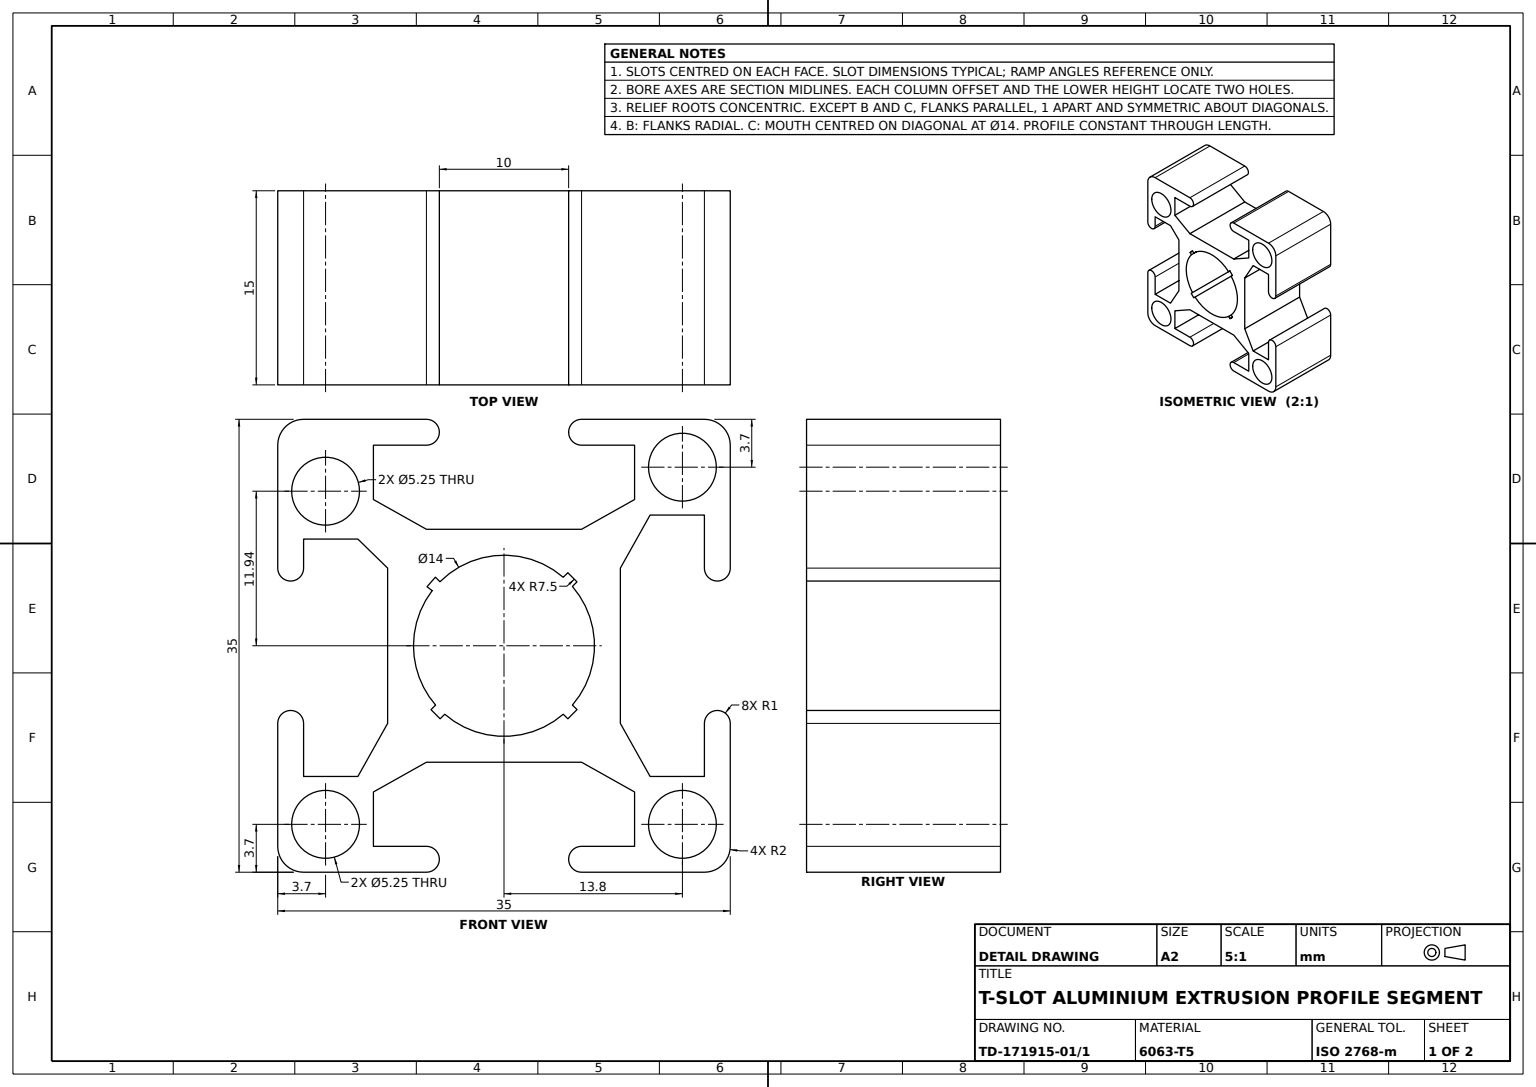
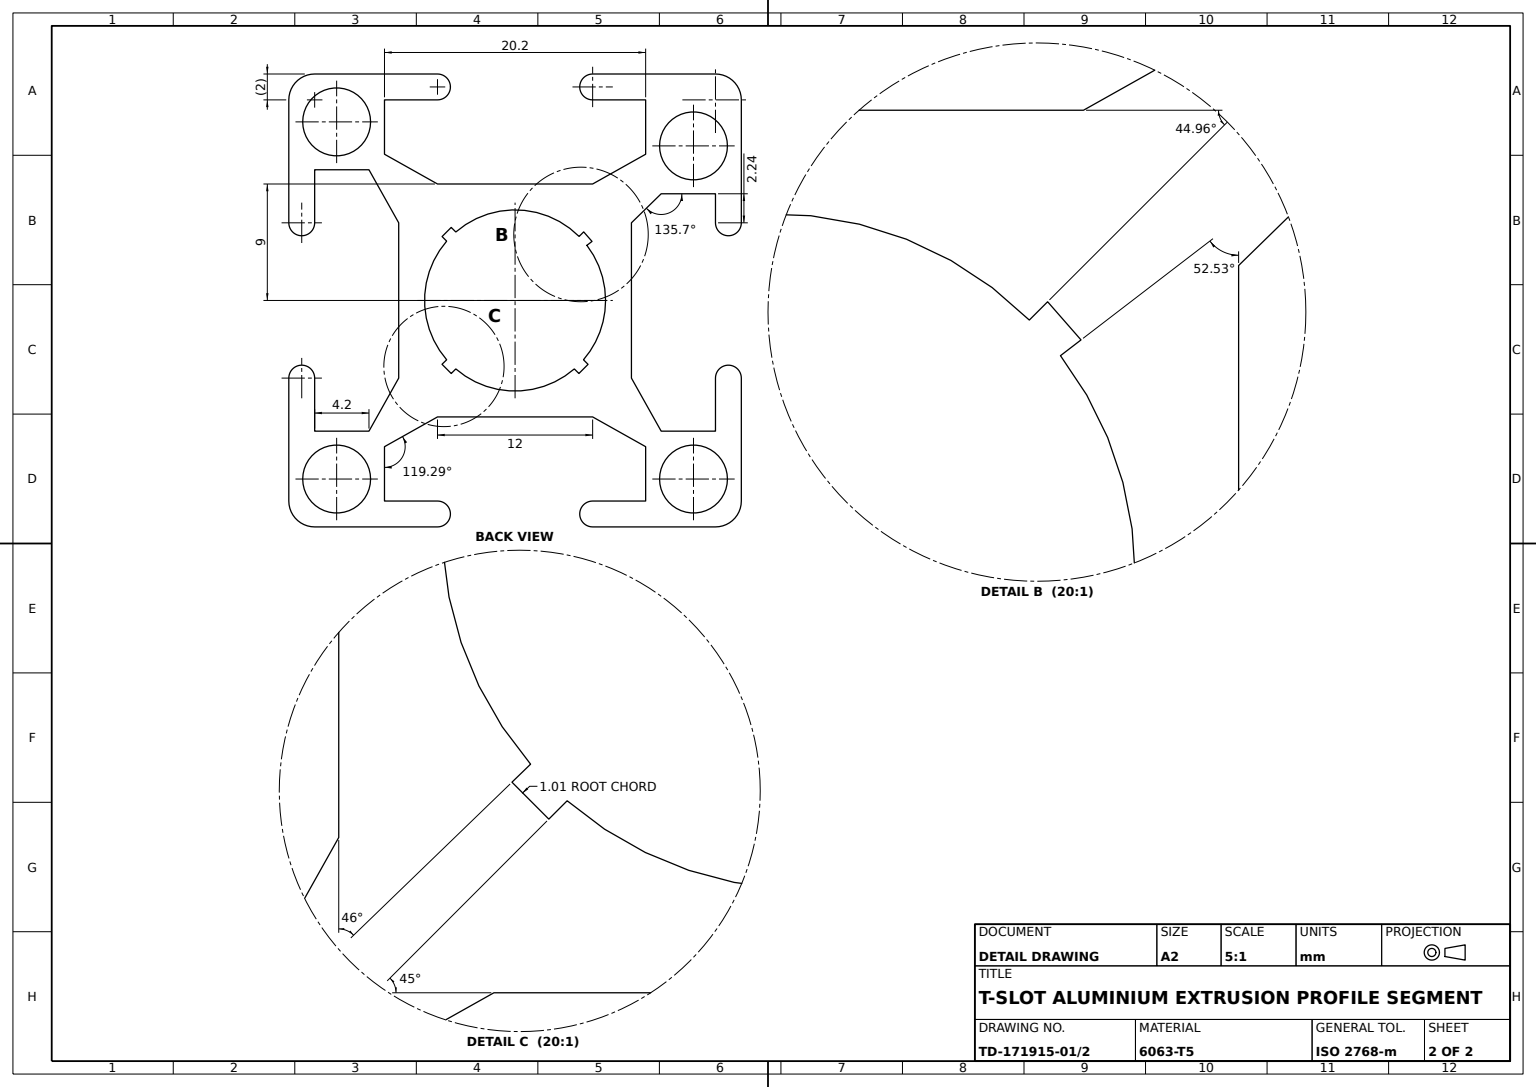
SolidWorks part; units mm, degrees
material "6063-T5"
ref_plane "Front Plane" through (0, 0, 0) normal (0, 0, 1) x (1, 0, 0)
ref_plane "Top Plane" through (0, 0, 0) normal (0, 1, 0) x (1, 0, 0)
ref_plane "Right Plane" through (0, 0, 0) normal (1, 0, 0) x (0, 0, -1)
sketch "Profile Section 35x35" plane through (0, 0, 0) normal (0, 0, 1) x (1, 0, 0)
  line L0 (0, -17.5) -> (-13.8, -17.5)
  line L1 (17.5, 0) -> (17.5, 15.5)
  line L2 (15.5, 17.5) -> (13.8, 17.5)
  line L3 (-17.5, 15.5) -> (-17.5, -15.5)
  line L4 (-15.5, -17.5) -> (15.5, -17.5)
  line L5 (17.5, -15.5) -> (17.5, 0)
  line L6 (13.8, 17.5) -> (6, 17.5)
  line L7 (15.5, 17.5) -> (13.8, 17.5)
  line L8 (6, 17.5) -> (-15.5, 17.5)
  line L9 (6, 17.5) -> (6, 16.5)
  line L10 (6, 15.5) -> (10.1, 15.5)
  line L11 (17.5, 15.5) -> (17.5, 6)
  line L12 (10.1, 11.3) -> (10.1, 15.5)
  line L13 (0, 17.5) -> (0, 9)
  line L15 (15.5, 6) -> (15.5, 10.1)
  line L16 (15.5, 10.1) -> (11.3, 10.1)
  line L17 (0, 9) -> (6, 9)
  line L18 (9, 6) -> (9, -6)
  line L19 (6, -9) -> (-6, -9)
  line L20 (-9, -6) -> (-9, 6)
  line L21 (-6, 9) -> (0, 9)
  line L22 (6, 9) -> (10.1, 11.3)
  line L23 (9, 6) -> (11.3, 10.1)
  line L24 (-15.5, -17.5) -> (-6, -17.5)
  line L25 (-17.5, -15.5) -> (-17.5, -6)
  line L26 (0, -9) -> (-6, -9)
  line L27 (-6, -15.5) -> (-10.1, -15.5)
  line L28 (-10.1, -15.5) -> (-10.1, -11.3)
  line L29 (-6, -9) -> (-10.1, -11.3)
  line L30 (-11.3, -10.1) -> (-15.5, -10.1)
  line L31 (-15.5, -10.1) -> (-15.5, -6)
  line L32 (-9, 0) -> (-9, -6)
  line L33 (-9, -6) -> (-11.3, -10.1)
  line L34 (15.5, -17.5) -> (6, -17.5)
  line L35 (6, -16.5) -> (6, -17.5)
  line L36 (0, -17.5) -> (13.8, -17.5)
  line L37 (9, 0) -> (9, -6)
  line L38 (10.1, -11.3) -> (10.1, -15.5)
  line L39 (10.1, -15.5) -> (6, -15.5)
  line L40 (17.5, -15.5) -> (17.5, -6)
  line L41 (17.5, -6) -> (16.5, -6)
  line L42 (9, -6) -> (11.3, -10.1)
  line L43 (15.5, -6) -> (15.5, -10.1)
  line L44 (15.5, -10.1) -> (11.3, -10.1)
  line L45 (0, -9) -> (6, -9)
  line L46 (6, -9) -> (10.1, -11.3)
  line L47 (-17.5, 15.5) -> (-17.5, 6)
  line L48 (-9, 0) -> (-9, 6)
  line L49 (0, 17.5) -> (-13.8, 17.5)
  line L50 (-11.3, 8.2442) -> (-15.5, 8.2442)
  line L51 (-15.5, 8.2442) -> (-15.5, 6)
  line L52 (-15.5, 17.5) -> (-6, 17.5)
  line L53 (-6, 17.5) -> (-6, 16.5)
  line L54 (-9, 6) -> (-11.3, 8.2442)
  line L55 (-10.1, 11.3) -> (-10.1, 15.5)
  line L56 (-10.1, 15.5) -> (-6, 15.5)
  line L57 (0, 9) -> (-6, 9)
  line L58 (-6, 9) -> (-10.1, 11.3)
  line L62 (5.2907, 4.5836) -> (5.6451, 4.9379)
  line L63 (4.5836, 5.2907) -> (4.9379, 5.6451)
  line L66 (5.2905, -4.5838) -> (5.6506, -4.9316)
  line L67 (-5.2907, -4.5836) -> (-5.6451, -4.9379)
  line L68 (4.5836, -5.2907) -> (4.9379, -5.6451)
  line L70 (-4.953, 4.9465) -> (-5.3068, 5.2998)
  line L71 (-4.5836, -5.2907) -> (-4.9379, -5.6451)
  line L72 (-5.5556, 4.2585) -> (-5.9525, 4.5627)
  circle A0 centre (-13.8, -13.8) radius 2.625
  arc A1 (15.5, -17.5) -> (17.5, -15.5) centre (15.5, -15.5) ccw
  arc A2 (-17.5, -15.5) -> (-15.5, -17.5) centre (-15.5, -15.5) ccw
  arc A3 (-15.5, 17.5) -> (-17.5, 15.5) centre (-15.5, 15.5) ccw
  arc A4 (17.5, 15.5) -> (15.5, 17.5) centre (15.5, 15.5) ccw
  circle A5 centre (13.8, 13.8) radius 2.625
  arc A6 (6, 17.5) -> (6, 15.5) centre (6, 16.5) ccw
  arc A7 (15.5, 6) -> (17.5, 6) centre (16.5, 6) ccw
  arc A8 (-5.5556, 4.2585) -> (-5.2907, -4.5836) centre (0, 0) ccw
  arc A9 (-6, -17.5) -> (-6, -15.5) centre (-6, -16.5) ccw
  arc A10 (-15.5, -6) -> (-17.5, -6) centre (-16.5, -6) ccw
  arc A11 (6, -15.5) -> (6, -17.5) centre (6, -16.5) ccw
  circle A12 centre (13.8, -13.8) radius 2.625
  arc A13 (17.5, -6) -> (15.5, -6) centre (16.5, -6) ccw
  arc A14 (-17.5, 6) -> (-15.5, 6) centre (-16.5, 6) ccw
  circle A15 centre (-13.8, 11.9442) radius 2.625
  arc A16 (-6, 15.5) -> (-6, 17.5) centre (-6, 16.5) ccw
  arc A18 (5.6451, 4.9379) -> (4.9379, 5.6451) centre (0, 0) ccw
  arc A19 (4.9379, -5.6451) -> (5.6506, -4.9316) centre (0, 0) ccw
  arc A20 (-5.6451, -4.9379) -> (-4.9379, -5.6451) centre (0, 0) ccw
  arc A21 (-5.3068, 5.2998) -> (-5.9525, 4.5627) centre (0, 0) ccw
  arc A22 (5.2905, -4.5838) -> (5.2907, 4.5836) centre (0, 0) ccw
  arc A23 (-4.5836, -5.2907) -> (4.5836, -5.2907) centre (0, 0) ccw
  arc A24 (4.5836, 5.2907) -> (-4.953, 4.9465) centre (0, 0) ccw
  point P13 (17.5, -17.5)
  point P16 (-17.5, -17.5)
  point P21 (17.5, 17.5)
  dimension "D6" = 2
  dimension "D7" = 7.8
  dimension "D8" = 5.25
  dimension "D9" = 5.25
  dimension "D10" = 13.8
  dimension "D13" = 1
  dimension "D16" = 12
  dimension "D18" = 5.25
  dimension "D19" = 3.7
  dimension "D20" = 9
  dimension "D33" = 14
  dimension "D34" = 15
  dimension "D1" = 17.5
  dimension "D2" = 17.5
  dimension "D3" = 35
  dimension "D4" = 17.5
  dimension "D5" = 17.5
  dimension "D11" = 19.5161
  dimension "D12" = 3.7
  dimension "D14" = 4.2
  dimension "D15" = 3.7
  dimension "D17" = 9
  dimension "D21" = 6
  dimension "D22" = 12
  dimension "D23" = 12
  dimension "D24" = 6
  dimension "D25" = 9
  dimension "D26" = 6
  dimension "D27" = 12
  dimension "D28" = 9
  dimension "D29" = 2.2442
  dimension "D30" = 3.7
  dimension "D31" = 3.7
  dimension "D32" = 11.9442
  dimension "D35" = 45
  dimension "D36" = 0.5
  dimension "D37" = 0.5
  dimension "D38" = 0.5
  dimension "D39" = 0.9997
  dimension "D40" = 1.0084
  dimension "D41" = 0.5
  dimension "D42" = 0.5
  dimension "D43" = 44.962
  dimension "D44" = 7.491
extrude "Profile Extrusion L15" add sketch "Profile Section 35x35" along normal mid plane 15
